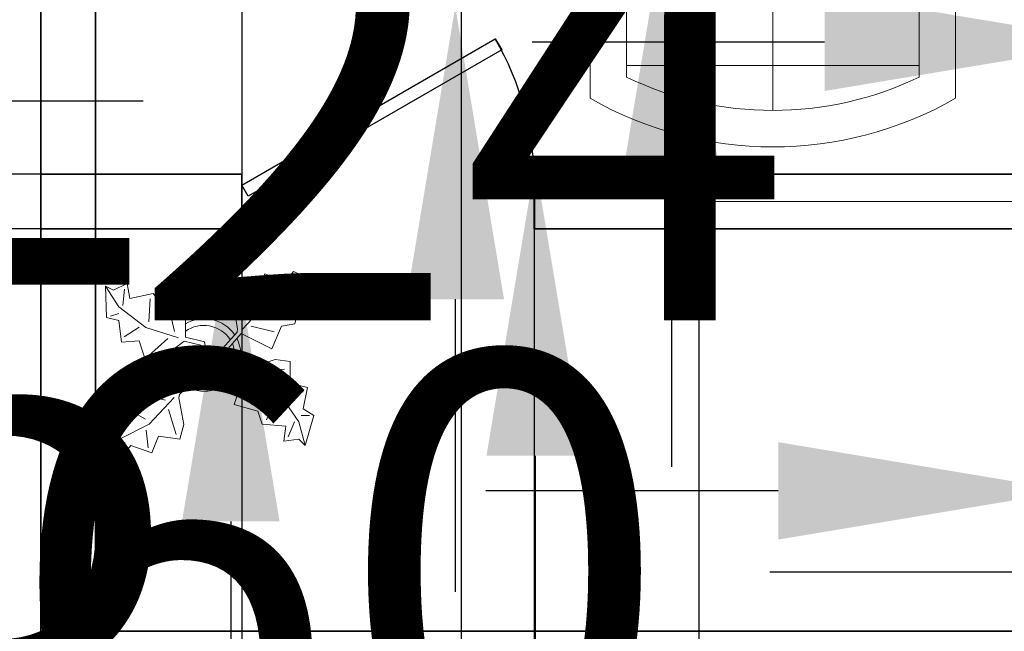
# Model space of a CAD drawing. Units: inches. Extents: x -307 to 2141, y -58 to 895.
# Tile 5 of 28: x 553 to 714, y 100 to 201. Entities that reach past the tile are written whole.
import ezdxf

# ---------------------------------------------------------------- set-up
doc = ezdxf.new("R2010")
doc.units = ezdxf.units.IN
doc.header["$MEASUREMENT"] = 0
for name, color, linetype, lineweight in [('A-ANNO-DIMS', 2, 'Continuous', 18), ('A-DOOR', 3, 'Continuous', 25), ('A-FURN', 8, 'Continuous', 18), ('A-GLAZ', 4, 'Continuous', 18), ('A-WALL', 7, 'Continuous', 35), ('L-PLNT', 94, 'Continuous', 13)]:
    doc.layers.add(name, color=color, linetype=linetype, lineweight=lineweight)
doc.styles.get("Standard").update_dxf_attribs({"font": 'arial.ttf'})
doc.dimstyles.get("Standard").update_dxf_attribs({"dimtxt": 72, "dimasz": 48, "dimexe": 0.18, "dimexo": 0.0625, "dimgap": 0.09, "dimtad": 0, "dimtih": 1, "dimtoh": 1, "dimdec": 0, "dimrnd": 48, "dimzin": 0, "dimdsep": 46, "dimlunit": 3, "dimtxsty": 'Standard', "dimcen": 0.09, "dimadec": 0, "dimazin": 0, "dimtfac": 1, "dimtdec": 0, "dimtofl": 0, "dimtmove": 0, "dimatfit": 3, "dimfxl": 1, "dimtolj": 1, "dimtzin": 0, "dimarcsym": 0})

# ---------------------------------------------------------------- blocks, each defined once
blk = doc.blocks.new('*U7')
for p, q in [((-40, 0), (-40, 6)), ((0, 0), (0, 6))]:
    blk.add_line(p, q)
blk.add_lwpolyline([(0, 0), (-34.64, -20), (-35.52, -18.48), (-0.88, 1.52)], close=True)
blk.add_arc((0, 0), 40, 180, 210)
blk = doc.blocks.new('Sofa - Roundback Loveseat 5 ft.')
for p, q in [((0, -32.44198), (0, -5.99998)), ((-24, -33.99998), (-24, -11.46958)), ((24.00004, -33.99998), (24.00004, -11.46958)), ((-23.9998, -13.38178), (23.99986, -13.38178)), ((-24, -32.44198), (24.00004, -32.44198))]:
    blk.add_line(p, q)
for points in [[(-24, -33.99998), (-30, -33.99998), (-30, -7.99998)], [(30.00004, -7.99998), (30.00004, -33.99998), (24.00004, -33.99998)]]:
    blk.add_lwpolyline(points)
for centre, radius, start, end in [((0, -60.24998), 60.24998, 60.13715, 119.8628), ((0, -61.38438), 55.38444, 64.32083, 115.6792)]:
    blk.add_arc(centre, radius, start, end)
blk = doc.blocks.new('Plant - Rubber or Philodendron')
for p, q in [((8.8871, 10.7908), (9.9809, 13.4933)), ((9.9809, 13.4933), (13.3837, 12.301)), ((13.3837, 12.301), (14.68, 13.9039)), ((14.5816, 13.2037), (14.3848, 11.8033)), ((14.68, 13.9039), (19.3848, 11.8146)), ((-16.2005, 11.4774), (-13.9899, 8.1064)), ((-16.2005, 11.4774), (-14.8639, 10.7964)), ((-16.0159, 6.3329), (-16.2005, 11.4774)), ((-14.8639, 10.7964), (-12.6195, 11.8975)), ((-12.6195, 11.8975), (-12.1909, 9.4345)), ((10.5828, 12.6946), (10.8893, 9.7953)), ((19.3848, 11.8146), (15.3859, 11.3055)), ((19.3848, 11.8146), (18.1868, 10.9119)), ((-13.3174, 8.325), (-13.0735, 11.0065)), ((-12.1909, 9.4345), (-8.3829, 10.3)), ((-8.3829, 10.3), (-7.0549, 8.501)), ((4.6914, 8.8812), (5.3859, 11.2828)), ((5.3859, 11.2828), (8.8871, 10.7908)), ((5.9878, 10.4842), (7.1971, 6.3869)), ((15.3859, 11.3055), (10.3916, 8.7942)), ((15.2875, 10.6053), (17.5907, 9.2105)), ((18.1868, 10.9119), (18.1925, 8.4119)), ((-13.9899, 8.1064), (-9.5434, 4.7185)), ((-8.8369, 9.409), (-9.0894, 5.6095)), ((-7.0549, 8.501), (-3.0284, 8.6941)), ((-3.0284, 8.6941), (-3.0709, 3.1041)), ((4.6914, 8.8812), (5.5014, 4.4831)), ((10.3916, 8.7942), (6.2847, 4.4028)), ((15.7909, 9.1065), (14.8995, 5.3044)), ((18.1925, 8.4119), (15.7909, 9.1065)), ((-15.3434, 6.5514), (-13.9984, 6.9884)), ((-4.8529, 4.012), (-5.7184, 7.82)), ((14.2977, 6.1031), (10.9934, 7.9956)), ((-14.0069, 5.8704), (-16.0159, 6.3329)), ((-13.5868, 2.2894), (-14.0069, 5.8704)), ((7.7005, 4.8881), (11.5025, 3.9967)), ((12.7005, 4.8994), (11.1089, 1.1958)), ((14.8995, 5.3044), (12.7005, 4.8994)), ((-13.1329, 3.1804), (-10.6614, 4.727)), ((-9.5434, 4.7185), (-4.1917, 2.9888)), ((2.1141, 0.2298), (5.4346, 3.9146)), ((6.1032, 3.6844), (2.8262, -0.031)), ((5.4346, 3.9146), (5.5014, 4.4831)), ((11.1089, 1.1958), (6.1032, 3.6844)), ((-10.6784, 2.491), (-13.5868, 2.2894)), ((-9.5858, -0.8715), (-10.6784, 2.491)), ((-9.1318, 0.0195), (-5.9793, 2.9025)), ((-7.1228, -0.443), (-3.5248, 2.2131)), ((-3.5248, 2.2131), (-3.3011, 2.4355)), ((-3.3011, 2.4355), (-0.5306, 1.7947)), ((-3.0709, 3.1041), (0.0797, 2.3163)), ((-0.5306, 1.7947), (-0.2255, -0.5527)), ((-0.5306, 1.7947), (-0.5306, 1.7947)), ((0.0797, 2.3163), (0.4866, -0.031)), ((0.4866, -0.031), (2.1141, 0.2298)), ((-7.1228, -0.443), (-9.5858, -0.8715)), ((-2.019, -3.6148), (-0.2255, -0.5527)), ((-0.9375, -3.1608), (0.5883, -0.8135)), ((0.5883, -0.8135), (2.2447, -2.0916)), ((2.8262, -0.031), (1.3003, -0.5527)), ((1.3003, -0.5527), (2.4193, -1.4655)), ((2.4193, -1.4655), (6.895, -2.1175)), ((11.6605, -0.5413), (6.895, -2.1175)), ((11.6605, -0.5413), (14.1354, -0.8948)), ((14.1354, -0.8948), (14.1354, -4.4304)), ((-4.0579, -6.2781), (-0.9375, -3.1608)), ((2.2447, -2.0916), (6.7108, -2.6626)), ((4.943, -7.9659), (6.7108, -2.6626)), ((12.3677, -6.1981), (7.219, -2.6772)), ((8.3544, -2.7453), (13.1973, -2.1704)), ((-11.3237, -7.2629), (-9.7321, -3.5593)), ((-9.7321, -3.5593), (-4.7264, -6.0479)), ((-2.019, -3.6148), (-4.7264, -6.0479)), ((8.125, -4.0768), (7.7715, -7.9659)), ((14.1354, -4.4304), (16.9638, -5.1375)), ((-6.3237, -7.2516), (-10.1257, -6.3602)), ((-4.1246, -6.8466), (-4.0579, -6.2781)), ((15.5496, -10.7943), (12.3677, -6.1981)), ((16.2567, -5.8446), (13.4283, -6.5517)), ((16.9638, -5.1375), (16.2567, -8.673)), ((-14.4141, -11.4699), (-13.5228, -7.6679)), ((-13.5228, -7.6679), (-11.3237, -7.2629)), ((-9.0148, -11.1577), (-4.9047, -6.8122)), ((-3.3146, -11.2447), (-4.1246, -6.8466)), ((8.8321, -9.0266), (4.943, -7.9659)), ((10.2463, -10.4408), (11.6605, -6.9053)), ((-12.921, -8.4665), (-9.6166, -10.359)), ((-4.611, -12.8477), (-5.8203, -8.7504)), ((9.5392, -11.1479), (8.8321, -9.0266)), ((16.2567, -8.673), (18.0245, -9.7337)), ((-16.8157, -10.7754), (-14.4141, -11.4699)), ((-16.8101, -13.2754), (-16.8157, -10.7754)), ((-14.0091, -13.669), (-9.0148, -11.1577)), ((-3.3146, -11.2447), (-4.0092, -13.6463)), ((13.4283, -11.5015), (9.5392, -11.1479)), ((14.8425, -10.7943), (13.7819, -13.2692)), ((16.6103, -14.6834), (15.5496, -10.7943)), ((17.3174, -9.7337), (15.9032, -9.7337)), ((18.0245, -9.7337), (16.6103, -14.6834)), ((-13.9107, -12.9688), (-16.2139, -11.574)), ((-9.206, -15.0581), (-9.5126, -12.1588)), ((13.0748, -13.9763), (13.4283, -11.5015)), ((-18.008, -14.1781), (-16.8101, -13.2754)), ((-18.008, -14.1781), (-14.0091, -13.669)), ((-13.3032, -16.2674), (-18.008, -14.1781)), ((-13.2048, -15.5672), (-13.008, -14.1668)), ((-7.5103, -13.1543), (-8.6042, -15.8568)), ((-4.0092, -13.6463), (-7.5103, -13.1543)), ((15.5496, -13.6228), (13.0748, -13.9763)), ((16.6103, -14.6834), (15.5496, -13.6228)), ((-12.0069, -14.6645), (-13.3032, -16.2674)), ((-8.6042, -15.8568), (-12.0069, -14.6645))]:
    blk.add_line(p, q)
for centre, radius, start, end in [((0, 0), 6.1275, 34.37569, 120.1028), ((-0.0601, -0.2075), 5.2461, 33.82192, 124.9414), ((-0.2664, 0.1682), 5.2775, 338.4094, 20.03007), ((-0.098, 0.1364), 6.1288, 341.2017, 26.09184), ((0.0308, 0.1664), 6, 178.6147, 235.1169), ((0.0308, 0.1664), 5, 168.1647, 238.6725), ((-0.0234, 0.3825), 6.1492, 242.5812, 331.2714), ((-0.1102, 0.4886), 5.2883, 247.3711, 327.472)]:
    blk.add_arc(centre, radius, start, end)
blk = doc.blocks.new('WIN-36IN-PAIR')
for p, q in [((72.02, 9), (72.02, 0)), ((0, 4.5), (36, 4.5)), ((36.02, 4.5), (72.02, 4.5))]:
    blk.add_line(p, q)
for points in [[(36, 0), (0, 0), (0, 9), (36, 9)], [(36.02, 9), (72.02, 9)], [(72.02, 0), (36.02, 0)]]:
    blk.add_lwpolyline(points)
blk = doc.blocks.new('*D28')
at = {"layer": 'A-ANNO-DIMS', "color": 0, "lineweight": -2, "transparency": 16777216}
for p, q in [((795.36, 433.55), (777.92, 433.55)), ((778.1, 385.55), (778.1, 366.07)), ((795.36, 318.07), (777.92, 318.07)), ((778.1, 318.07), (778.1, 270.07)), ((778.1, 270.07), (730.1, 270.07))]:
    blk.add_line(p, q, dxfattribs=at)
at = {"layer": 'A-ANNO-DIMS', "color": 0, "transparency": 16777216}
for points in [[(770.1, 385.55), (786.1, 385.55), (778.1, 433.55)], [(770.1, 366.07), (786.1, 366.07), (778.1, 318.07)]]:
    blk.add_solid(points, dxfattribs=at)
at = {"layer": 'Defpoints', "color": 0, "transparency": 16777216}
for p in [(795.42, 433.55), (778.1, 318.07), (795.42, 318.07)]:
    blk.add_point(p, dxfattribs=at)
at = {"layer": 'A-ANNO-DIMS', "color": 0, "transparency": 16777216, "insert": (534.42, 270.07), "char_height": 72, "attachment_point": 5}
blk.add_mtext('\\A1;BED 115', dxfattribs=at)
blk = doc.blocks.new('*D38')
at = {"layer": 'A-ANNO-DIMS', "color": 0, "lineweight": -2, "transparency": 16777216}
for p, q in [((598.5, 222.79), (550.5, 222.79)), ((646.5, 213.85), (646.5, 222.97)), ((706.5, 213.85), (706.5, 222.97)), ((754.5, 222.79), (802.5, 222.79))]:
    blk.add_line(p, q, dxfattribs=at)
at = {"layer": 'A-ANNO-DIMS', "color": 0, "transparency": 16777216}
for points in [[(598.5, 230.79), (598.5, 214.79), (646.5, 222.79)], [(754.5, 230.79), (754.5, 214.79), (706.5, 222.79)]]:
    blk.add_solid(points, dxfattribs=at)
at = {"layer": 'Defpoints', "color": 0, "transparency": 16777216}
for p in [(646.5, 222.79), (646.5, 213.79), (706.5, 213.79)]:
    blk.add_point(p, dxfattribs=at)
at = {"layer": 'A-ANNO-DIMS', "color": 0, "transparency": 16777216, "insert": (97.26, 222.79), "char_height": 72, "attachment_point": 5}
blk.add_mtext('\\A1;LOVESEAT 60 TYP.', dxfattribs=at)
blk = doc.blocks.new('*D39')
at = {"layer": 'A-ANNO-DIMS', "color": 0, "lineweight": -2, "transparency": 16777216}
for p, q in [((637.5, 261.79), (637.5, 309.79)), ((646.43, 213.79), (637.32, 213.79)), ((646.43, 177.12), (637.32, 177.12)), ((637.5, 129.12), (637.5, 81.12)), ((637.5, 81.12), (589.5, 81.12))]:
    blk.add_line(p, q, dxfattribs=at)
at = {"layer": 'A-ANNO-DIMS', "color": 0, "transparency": 16777216}
for points in [[(629.5, 261.79), (645.5, 261.79), (637.5, 213.79)], [(629.5, 129.12), (645.5, 129.12), (637.5, 177.12)]]:
    blk.add_solid(points, dxfattribs=at)
at = {"layer": 'Defpoints', "color": 0, "transparency": 16777216}
for p in [(646.5, 213.79), (637.5, 177.12), (646.5, 177.12)]:
    blk.add_point(p, dxfattribs=at)
at = {"layer": 'A-ANNO-DIMS', "color": 0, "transparency": 16777216, "insert": (414.2, 81.12), "char_height": 72, "attachment_point": 5}
blk.add_mtext('\\A1;37 TYP.', dxfattribs=at)
blk = doc.blocks.new('*D40')
at = {"layer": 'A-ANNO-DIMS', "color": 0, "lineweight": -2, "transparency": 16777216}
for p, q in [((725.38, 128.89), (725.38, 123.17)), ((762.77, 128.89), (762.77, 123.17)), ((677.38, 123.35), (629.38, 123.35)), ((810.77, 123.35), (858.77, 123.35))]:
    blk.add_line(p, q, dxfattribs=at)
at = {"layer": 'A-ANNO-DIMS', "color": 0, "transparency": 16777216}
for points in [[(677.38, 131.35), (677.38, 115.35), (725.38, 123.35)], [(810.77, 131.35), (810.77, 115.35), (762.77, 123.35)]]:
    blk.add_solid(points, dxfattribs=at)
at = {"layer": 'Defpoints', "color": 0, "transparency": 16777216}
for p in [(725.38, 128.96), (762.77, 128.96), (762.77, 123.35)]:
    blk.add_point(p, dxfattribs=at)
at = {"layer": 'A-ANNO-DIMS', "color": 0, "transparency": 16777216, "insert": (1208.37, 123.35), "char_height": 72, "attachment_point": 5}
blk.add_mtext('\\A1;PLANT 37 TYP.', dxfattribs=at)
blk = doc.blocks.new('*D48')
at = {"layer": 'A-ANNO-DIMS', "color": 0, "lineweight": -2, "transparency": 16777216}
for p, q in [((724, 313.98), (724, 361.98)), ((732.94, 265.98), (723.82, 265.98)), ((732.94, 205.98), (723.82, 205.98)), ((724, 157.98), (724, 109.98)), ((724, 109.98), (676, 109.98))]:
    blk.add_line(p, q, dxfattribs=at)
at = {"layer": 'A-ANNO-DIMS', "color": 0, "transparency": 16777216}
for points in [[(716, 313.98), (732, 313.98), (724, 265.98)], [(716, 157.98), (732, 157.98), (724, 205.98)]]:
    blk.add_solid(points, dxfattribs=at)
at = {"layer": 'Defpoints', "color": 0, "transparency": 16777216}
for p in [(733, 265.98), (724, 205.98), (733, 205.98)]:
    blk.add_point(p, dxfattribs=at)
at = {"layer": 'A-ANNO-DIMS', "color": 0, "transparency": 16777216, "insert": (321.56, 109.98), "char_height": 72, "attachment_point": 5}
blk.add_mtext('\\A1;MEDIA UNIT 60', dxfattribs=at)
blk = doc.blocks.new('*D49')
at = {"layer": 'A-ANNO-DIMS', "color": 0, "lineweight": -2, "transparency": 16777216}
for p, q in [((733, 205.92), (733, 196.8)), ((754.34, 205.92), (754.34, 196.8)), ((685, 196.98), (637, 196.98)), ((802.34, 196.98), (850.34, 196.98))]:
    blk.add_line(p, q, dxfattribs=at)
at = {"layer": 'A-ANNO-DIMS', "color": 0, "transparency": 16777216}
for points in [[(685, 204.98), (685, 188.98), (733, 196.98)], [(802.34, 204.98), (802.34, 188.98), (754.34, 196.98)]]:
    blk.add_solid(points, dxfattribs=at)
at = {"layer": 'Defpoints', "color": 0, "transparency": 16777216}
for p in [(733, 205.98), (754.34, 205.98), (754.34, 196.98)]:
    blk.add_point(p, dxfattribs=at)
at = {"layer": 'A-ANNO-DIMS', "color": 0, "transparency": 16777216, "insert": (895.66, 196.98), "char_height": 72, "attachment_point": 5}
blk.add_mtext('\\A1;21', dxfattribs=at)
blk = doc.blocks.new('*D58')
at = {"layer": 'A-ANNO-DIMS', "color": 0, "lineweight": -2, "transparency": 16777216}
for p, q in [((624.38, 334.8), (624.38, 382.8)), ((611.84, 286.8), (624.56, 286.8)), ((611.84, 202.8), (624.56, 202.8)), ((624.38, 154.8), (624.38, 106.8))]:
    blk.add_line(p, q, dxfattribs=at)
at = {"layer": 'A-ANNO-DIMS', "color": 0, "transparency": 16777216}
for points in [[(616.38, 334.8), (632.38, 334.8), (624.38, 286.8)], [(616.38, 154.8), (632.38, 154.8), (624.38, 202.8)]]:
    blk.add_solid(points, dxfattribs=at)
at = {"layer": 'Defpoints', "color": 0, "transparency": 16777216}
for p in [(611.78, 286.8), (624.38, 286.8), (611.78, 202.8)]:
    blk.add_point(p, dxfattribs=at)
at = {"layer": 'A-ANNO-DIMS', "color": 0, "transparency": 16777216, "insert": (624.38, 244.8), "char_height": 72, "attachment_point": 5}
blk.add_mtext('\\A1;SOFA 84', dxfattribs=at)
blk = doc.blocks.new('*D60')
at = {"layer": 'A-ANNO-DIMS', "color": 0, "lineweight": -2, "transparency": 16777216}
for p, q in [((659.86, 294.95), (659.86, 342.95)), ((659.86, 342.95), (707.86, 342.95)), ((663.34, 246.95), (659.68, 246.95)), ((663.34, 223.32), (659.68, 223.32)), ((659.86, 175.32), (659.86, 127.32))]:
    blk.add_line(p, q, dxfattribs=at)
at = {"layer": 'A-ANNO-DIMS', "color": 0, "transparency": 16777216}
for points in [[(651.86, 294.95), (667.86, 294.95), (659.86, 246.95)], [(651.86, 175.32), (667.86, 175.32), (659.86, 223.32)]]:
    blk.add_solid(points, dxfattribs=at)
at = {"layer": 'Defpoints', "color": 0, "transparency": 16777216}
for p in [(659.86, 246.95), (663.4, 246.95), (663.4, 223.32)]:
    blk.add_point(p, dxfattribs=at)
at = {"layer": 'A-ANNO-DIMS', "color": 0, "transparency": 16777216, "insert": (933.57, 342.95), "char_height": 72, "attachment_point": 5}
blk.add_mtext('\\A1;TABLE 24', dxfattribs=at)
blk = doc.blocks.new('*D63')
at = {"layer": 'A-ANNO-DIMS', "color": 0, "lineweight": -2, "transparency": 16777216}
for p, q in [((916.4, 691.34), (947.72, 691.34)), ((947.54, 643.34), (947.54, 416.19)), ((947.54, 115.34), (947.54, 342.49)), ((704.68, 67.34), (947.72, 67.34))]:
    blk.add_line(p, q, dxfattribs=at)
at = {"layer": 'A-ANNO-DIMS', "color": 0, "transparency": 16777216}
for points in [[(939.54, 643.34), (955.54, 643.34), (947.54, 691.34)], [(939.54, 115.34), (955.54, 115.34), (947.54, 67.34)]]:
    blk.add_solid(points, dxfattribs=at)
at = {"layer": 'Defpoints', "color": 0, "transparency": 16777216}
for p in [(916.34, 691.34), (704.62, 67.34), (947.54, 67.34)]:
    blk.add_point(p, dxfattribs=at)
at = {"layer": 'A-ANNO-DIMS', "color": 0, "transparency": 16777216, "insert": (947.54, 379.34), "char_height": 72, "attachment_point": 5}
blk.add_mtext('\\A1;624', dxfattribs=at)
blk = doc.blocks.new('*D64')
at = {"layer": 'A-ANNO-DIMS', "color": 0, "lineweight": -2, "transparency": 16777216}
for p, q in [((556.27, 691.34), (524.95, 691.34)), ((525.13, 643.34), (525.13, 465.69)), ((525.13, 214.34), (525.13, 391.99)), ((556.27, 166.34), (524.95, 166.34))]:
    blk.add_line(p, q, dxfattribs=at)
at = {"layer": 'A-ANNO-DIMS', "color": 0, "transparency": 16777216}
for points in [[(517.13, 643.34), (533.13, 643.34), (525.13, 691.34)], [(517.13, 214.34), (533.13, 214.34), (525.13, 166.34)]]:
    blk.add_solid(points, dxfattribs=at)
at = {"layer": 'Defpoints', "color": 0, "transparency": 16777216}
for p in [(525.13, 691.34), (556.34, 691.34), (556.34, 166.34)]:
    blk.add_point(p, dxfattribs=at)
at = {"layer": 'A-ANNO-DIMS', "color": 0, "transparency": 16777216, "insert": (525.13, 428.84), "char_height": 72, "attachment_point": 5}
blk.add_mtext('\\A1;525', dxfattribs=at)
blk = doc.blocks.new('*D65')
at = {"layer": 'A-ANNO-DIMS', "color": 0, "lineweight": -2, "transparency": 16777216}
for p, q in [((587.54, 252.57), (587.54, 300.57)), ((556.4, 204.57), (587.72, 204.57)), ((556.4, 166.34), (587.72, 166.34)), ((587.54, 118.34), (587.54, 70.34)), ((587.54, 70.34), (539.54, 70.34))]:
    blk.add_line(p, q, dxfattribs=at)
at = {"layer": 'A-ANNO-DIMS', "color": 0, "transparency": 16777216}
for points in [[(579.54, 252.57), (595.54, 252.57), (587.54, 204.57)], [(579.54, 118.34), (595.54, 118.34), (587.54, 166.34)]]:
    blk.add_solid(points, dxfattribs=at)
at = {"layer": 'Defpoints', "color": 0, "transparency": 16777216}
for p in [(556.34, 204.57), (556.34, 166.34), (587.54, 166.34)]:
    blk.add_point(p, dxfattribs=at)
at = {"layer": 'A-ANNO-DIMS', "color": 0, "transparency": 16777216, "insert": (417.99, 70.34), "char_height": 72, "attachment_point": 5}
blk.add_mtext('\\A1;38.23', dxfattribs=at)
blk = doc.blocks.new('*D66')
at = {"layer": 'A-ANNO-DIMS', "color": 0, "lineweight": -2, "transparency": 16777216}
for p, q in [((525.13, 382.34), (525.13, 430.34)), ((556.27, 334.34), (524.95, 334.34)), ((565.27, 304.34), (524.95, 304.34)), ((525.13, 256.34), (525.13, 208.34)), ((525.13, 208.34), (477.13, 208.34))]:
    blk.add_line(p, q, dxfattribs=at)
at = {"layer": 'A-ANNO-DIMS', "color": 0, "transparency": 16777216}
for points in [[(517.13, 382.34), (533.13, 382.34), (525.13, 334.34)], [(517.13, 256.34), (533.13, 256.34), (525.13, 304.34)]]:
    blk.add_solid(points, dxfattribs=at)
at = {"layer": 'Defpoints', "color": 0, "transparency": 16777216}
for p in [(556.34, 334.34), (525.13, 304.34), (565.34, 304.34)]:
    blk.add_point(p, dxfattribs=at)
at = {"layer": 'A-ANNO-DIMS', "color": 0, "transparency": 16777216, "insert": (425.62, 208.34), "char_height": 72, "attachment_point": 5}
blk.add_mtext('\\A1;30', dxfattribs=at)
blk = doc.blocks.new('*D70')
at = {"layer": 'A-ANNO-DIMS', "color": 0, "lineweight": -2, "transparency": 16777216}
for p, q in [((525.13184, 214.340828), (525.13184, 262.340828)), ((556.27334, 166.340828), (524.95184, 166.340828)), ((556.27334, 91.340828), (524.95184, 91.340828)), ((525.13184, 43.340828), (525.13184, -4.659172))]:
    blk.add_line(p, q, dxfattribs=at)
at = {"layer": 'A-ANNO-DIMS', "color": 0, "transparency": 16777216}
for points in [[(517.13184, 214.340828), (533.13184, 214.340828), (525.13184, 166.340828)], [(517.13184, 43.340828), (533.13184, 43.340828), (525.13184, 91.340828)]]:
    blk.add_solid(points, dxfattribs=at)
at = {"layer": 'Defpoints', "color": 0, "transparency": 16777216}
for p in [(525.13184, 166.340828), (556.33584, 166.340828), (556.33584, 91.340828)]:
    blk.add_point(p, dxfattribs=at)
at = {"layer": 'A-ANNO-DIMS', "color": 0, "transparency": 16777216, "insert": (525.13184, 128.840828), "char_height": 72, "attachment_point": 5}
blk.add_mtext('\\A1;75', dxfattribs=at)
blk = doc.blocks.new('*D71')
at = {"layer": 'A-ANNO-DIMS', "color": 0, "lineweight": -2, "transparency": 16777216}
for p, q in [((525.13, 139.34), (525.13, 187.34)), ((525.13, 187.34), (573.13, 187.34)), ((632.56, 91.34), (524.95, 91.34)), ((632.56, 67.34), (524.95, 67.34)), ((525.13, 19.34), (525.13, -28.66))]:
    blk.add_line(p, q, dxfattribs=at)
at = {"layer": 'A-ANNO-DIMS', "color": 0, "transparency": 16777216}
for points in [[(517.13, 139.34), (533.13, 139.34), (525.13, 91.34)], [(517.13, 19.34), (533.13, 19.34), (525.13, 67.34)]]:
    blk.add_solid(points, dxfattribs=at)
at = {"layer": 'Defpoints', "color": 0, "transparency": 16777216}
for p in [(525.13, 91.34), (632.62, 91.34), (632.62, 67.34)]:
    blk.add_point(p, dxfattribs=at)
at = {"layer": 'A-ANNO-DIMS', "color": 0, "transparency": 16777216, "insert": (625.26, 187.34), "char_height": 72, "attachment_point": 5}
blk.add_mtext('\\A1;24', dxfattribs=at)
blk = doc.blocks.new('*D86')
at = {"layer": 'A-ANNO-DIMS', "color": 0, "lineweight": -2, "transparency": 16777216}
for p, q in [((565.34, 304.28), (565.34, 35.96)), ((625.34, 304.28), (625.34, 35.96)), ((517.34, 36.14), (469.34, 36.14)), ((673.34, 36.14), (721.34, 36.14))]:
    blk.add_line(p, q, dxfattribs=at)
at = {"layer": 'A-ANNO-DIMS', "color": 0, "transparency": 16777216}
for points in [[(517.34, 44.14), (517.34, 28.14), (565.34, 36.14)], [(673.34, 44.14), (673.34, 28.14), (625.34, 36.14)]]:
    blk.add_solid(points, dxfattribs=at)
at = {"layer": 'Defpoints', "color": 0, "transparency": 16777216}
for p in [(565.34, 304.34), (625.34, 304.34), (625.34, 36.14)]:
    blk.add_point(p, dxfattribs=at)
at = {"layer": 'A-ANNO-DIMS', "color": 0, "transparency": 16777216, "insert": (773.07, 36.14), "char_height": 72, "attachment_point": 5}
blk.add_mtext('\\A1;60', dxfattribs=at)
blk = doc.blocks.new('*D89')
at = {"layer": 'A-ANNO-DIMS', "color": 0, "lineweight": -2, "transparency": 16777216}
for p, q in [((525.13, 295.34), (525.13, 343.34)), ((525.13, 343.34), (573.13, 343.34)), ((565.27, 295.34), (524.95, 295.34)), ((525.13, 223.34), (525.13, 247.34)), ((556.27, 175.34), (524.95, 175.34))]:
    blk.add_line(p, q, dxfattribs=at)
at = {"layer": 'A-ANNO-DIMS', "color": 0, "transparency": 16777216}
for points in [[(517.13, 247.34), (533.13, 247.34), (525.13, 295.34)], [(517.13, 223.34), (533.13, 223.34), (525.13, 175.34)]]:
    blk.add_solid(points, dxfattribs=at)
at = {"layer": 'Defpoints', "color": 0, "transparency": 16777216}
for p in [(525.13, 295.34), (565.34, 295.34), (556.34, 175.34)]:
    blk.add_point(p, dxfattribs=at)
at = {"layer": 'A-ANNO-DIMS', "color": 0, "transparency": 16777216, "insert": (649.25, 343.34), "char_height": 72, "attachment_point": 5}
blk.add_mtext('\\A1;120', dxfattribs=at)
blk = doc.blocks.new('*D90')
at = {"layer": 'A-ANNO-DIMS', "color": 0, "lineweight": -2, "transparency": 16777216}
for p, q in [((556.34, 166.28), (556.34, 35.96)), ((589.34, 166.28), (589.34, 35.96)), ((508.34, 36.14), (460.34, 36.14)), ((637.34, 36.14), (685.34, 36.14))]:
    blk.add_line(p, q, dxfattribs=at)
at = {"layer": 'A-ANNO-DIMS', "color": 0, "transparency": 16777216}
for points in [[(508.34, 44.14), (508.34, 28.14), (556.34, 36.14)], [(637.34, 44.14), (637.34, 28.14), (589.34, 36.14)]]:
    blk.add_solid(points, dxfattribs=at)
at = {"layer": 'Defpoints', "color": 0, "transparency": 16777216}
for p in [(556.34, 166.34), (589.34, 166.34), (589.34, 36.14)]:
    blk.add_point(p, dxfattribs=at)
at = {"layer": 'A-ANNO-DIMS', "color": 0, "transparency": 16777216, "insert": (736.97, 36.14), "char_height": 72, "attachment_point": 5}
blk.add_mtext('\\A1;33', dxfattribs=at)
blk = doc.blocks.new('*D91')
at = {"layer": 'A-ANNO-DIMS', "color": 0, "lineweight": -2, "transparency": 16777216}
for p, q in [((589.34, 166.28), (589.34, 35.96)), ((637.34, 166.28), (637.34, 35.96)), ((541.34, 36.14), (493.34, 36.14)), ((685.34, 36.14), (733.34, 36.14))]:
    blk.add_line(p, q, dxfattribs=at)
at = {"layer": 'A-ANNO-DIMS', "color": 0, "transparency": 16777216}
for points in [[(541.34, 44.14), (541.34, 28.14), (589.34, 36.14)], [(685.34, 44.14), (685.34, 28.14), (637.34, 36.14)]]:
    blk.add_solid(points, dxfattribs=at)
at = {"layer": 'Defpoints', "color": 0, "transparency": 16777216}
for p in [(589.34, 166.34), (637.34, 166.34), (637.34, 36.14)]:
    blk.add_point(p, dxfattribs=at)
at = {"layer": 'A-ANNO-DIMS', "color": 0, "transparency": 16777216, "insert": (786.52, 36.14), "char_height": 72, "attachment_point": 5}
blk.add_mtext('\\A1;48', dxfattribs=at)
blk = doc.blocks.new('*D92')
at = {"layer": 'A-ANNO-DIMS', "color": 0, "lineweight": -2, "transparency": 16777216}
for p, q in [((637.34, 166.28), (637.34, 35.96)), ((664.34, 166.28), (664.34, 35.96)), ((589.34, 36.14), (541.34, 36.14)), ((712.34, 36.14), (760.34, 36.14))]:
    blk.add_line(p, q, dxfattribs=at)
at = {"layer": 'A-ANNO-DIMS', "color": 0, "transparency": 16777216}
for points in [[(589.34, 44.14), (589.34, 28.14), (637.34, 36.14)], [(712.34, 44.14), (712.34, 28.14), (664.34, 36.14)]]:
    blk.add_solid(points, dxfattribs=at)
at = {"layer": 'Defpoints', "color": 0, "transparency": 16777216}
for p in [(637.34, 166.34), (664.34, 166.34), (664.34, 36.14)]:
    blk.add_point(p, dxfattribs=at)
at = {"layer": 'A-ANNO-DIMS', "color": 0, "transparency": 16777216, "insert": (812.61, 36.14), "char_height": 72, "attachment_point": 5}
blk.add_mtext('\\A1;27', dxfattribs=at)
blk = doc.blocks.new('*D99')
at = {"layer": 'A-ANNO-DIMS', "color": 0, "lineweight": -2, "transparency": 16777216}
for p, q in [((763.34, 481.28), (763.34, 35.96)), ((802.34, 481.28), (802.34, 35.96)), ((715.34, 36.14), (667.34, 36.14)), ((850.34, 36.14), (898.34, 36.14))]:
    blk.add_line(p, q, dxfattribs=at)
at = {"layer": 'A-ANNO-DIMS', "color": 0, "transparency": 16777216}
for points in [[(715.34, 44.14), (715.34, 28.14), (763.34, 36.14)], [(850.34, 44.14), (850.34, 28.14), (802.34, 36.14)]]:
    blk.add_solid(points, dxfattribs=at)
at = {"layer": 'Defpoints', "color": 0, "transparency": 16777216}
for p in [(763.34, 481.34), (802.34, 481.34), (802.34, 36.14)]:
    blk.add_point(p, dxfattribs=at)
at = {"layer": 'A-ANNO-DIMS', "color": 0, "transparency": 16777216, "insert": (950.04, 36.14), "char_height": 72, "attachment_point": 5}
blk.add_mtext('\\A1;39', dxfattribs=at)
blk = doc.blocks.new('*D100')
at = {"layer": 'A-ANNO-DIMS', "color": 0, "lineweight": -2, "transparency": 16777216}
for p, q in [((589.34, 409.28), (589.34, 35.96)), ((625.34, 409.28), (625.34, 35.96)), ((541.34, 36.14), (493.34, 36.14)), ((673.34, 36.14), (721.34, 36.14))]:
    blk.add_line(p, q, dxfattribs=at)
at = {"layer": 'A-ANNO-DIMS', "color": 0, "transparency": 16777216}
for points in [[(541.34, 44.14), (541.34, 28.14), (589.34, 36.14)], [(673.34, 44.14), (673.34, 28.14), (625.34, 36.14)]]:
    blk.add_solid(points, dxfattribs=at)
at = {"layer": 'Defpoints', "color": 0, "transparency": 16777216}
for p in [(589.34, 409.34), (625.34, 409.34), (625.34, 36.14)]:
    blk.add_point(p, dxfattribs=at)
at = {"layer": 'A-ANNO-DIMS', "color": 0, "transparency": 16777216, "insert": (772.95, 36.14), "char_height": 72, "attachment_point": 5}
blk.add_mtext('\\A1;36', dxfattribs=at)

msp = doc.modelspace()

# ---------------------------------------------------------------- linework, layer by layer
at = {"layer": 'A-WALL'}
for p, q in [((556.3358, 691.3408), (556.3358, 91.3408)), ((565.3358, 682.3408), (565.3358, 100.3408)), ((589.3358, 175.3408), (556.3358, 175.3408)), ((589.3358, 175.3408), (589.3358, 166.3408)), ((754.3358, 175.3408), (637.3358, 175.3408)), ((637.3358, 175.3408), (637.3358, 166.3408)), ((589.3358, 166.3408), (556.3358, 166.3408)), ((763.3358, 166.3408), (637.3358, 166.3408)), ((565.3358, 100.3408), (763.3358, 100.3408))]:
    msp.add_line(p, q, dxfattribs=at)

# ---------------------------------------------------------------- block references
at = {"layer": 'A-DOOR', "xscale": 1.201029199664418, "yscale": 1.201029199664418, "zscale": 1.201029199664418, "rotation": 179.9999999999999}
msp.add_blockref('*U7', (589.3358, 173.547), dxfattribs=at)
at = {"layer": 'A-FURN', "rotation": 180}
msp.add_blockref('Sofa - Roundback Loveseat 5 ft.', (676.4965, 179.7908), dxfattribs=at)
at = {"layer": 'A-GLAZ'}
msp.add_blockref('WIN-36IN-PAIR', (664.336, 166.341), dxfattribs=at)
at = {"layer": 'L-PLNT'}
msp.add_blockref('Plant - Rubber or Philodendron', (583.1583, 145.4681), dxfattribs=at)

# ---------------------------------------------------------------- dimensions: what is measured, and where the dimension line sits
at = {"layer": 'A-ANNO-DIMS'}
for base, p1, p2, angle, override, picture, middle in [((525.1318, 691.3408), (556.3358, 166.3408), (556.3358, 691.3408), 90, {"dimdec": 0, "dimlfac": 1, "dimrnd": 0, "dimzin": 0, "dimdsep": 46, "dimlunit": 2}, '*D64', (525.1318, 428.8408)), ((947.5398, 67.3408), (916.3358, 691.3408), (704.6211, 67.3408), 90, {"dimdec": 0, "dimlfac": 1, "dimrnd": 0, "dimzin": 0, "dimdsep": 46, "dimlunit": 2}, '*D63', (947.5398, 379.3408)), ((525.1318, 304.3408), (556.3358, 334.3416), (565.3358, 304.3408), 90, {"dimdec": 0, "dimlfac": 1, "dimrnd": 0, "dimzin": 0, "dimdsep": 46, "dimlunit": 2}, '*D66', (425.6203, 208.3408)), ((525.1318, 295.3408), (556.3358, 175.3408), (565.3358, 295.3408), 90, {"dimdec": 0, "dimlfac": 1, "dimrnd": 0, "dimzin": 0, "dimdsep": 46, "dimlunit": 2}, '*D89', (649.2491, 343.3408)), ((587.5398, 166.3408), (556.3358, 204.574), (556.3358, 166.3408), 270, {"dimdec": 2, "dimlfac": 1, "dimrnd": 0, "dimzin": 0, "dimdsep": 46, "dimlunit": 2}, '*D65', (417.9928, 70.3408)), ((525.1318, 166.3408), (556.3358, 91.3408), (556.3358, 166.3408), 90, {"dimdec": 0, "dimlfac": 1, "dimrnd": 0, "dimzin": 0, "dimdsep": 46, "dimlunit": 2}, '*D70', (525.1318, 128.8408)), ((525.1318, 91.3408), (632.6211, 67.3408), (632.6211, 91.3408), 90, {"dimdec": 0, "dimlfac": 1, "dimrnd": 0, "dimzin": 0, "dimdsep": 46, "dimlunit": 2}, '*D71', (625.2573, 187.3408))]:
    dim = msp.add_linear_dim(base=base, p1=p1, p2=p2, angle=angle, dimstyle='Standard', override=override, dxfattribs=at)
    dim.commit()
    dim.dimension.update_dxf_attribs({"geometry": picture, "text_midpoint": middle})
for base, p1, p2, picture, middle in [((802.3358, 36.1368), (763.3358, 481.3408), (802.3358, 481.3408), '*D99', (950.0438, 36.1368)), ((625.3358, 36.1368), (589.339, 409.3408), (625.3358, 409.3408), '*D100', (772.9456, 36.1368)), ((625.3358, 36.1368), (565.3358, 304.3408), (625.3358, 304.3408), '*D86', (773.0684, 36.1368)), ((754.3358, 196.9815), (733.0025, 205.9815), (754.3358, 205.9815), '*D49', (895.6591, 196.9815)), ((589.3358, 36.1368), (556.3358, 166.3408), (589.3358, 166.3408), '*D90', (736.9702, 36.1368)), ((637.3358, 36.1368), (589.3358, 166.3408), (637.3358, 166.3408), '*D91', (786.5172, 36.1368)), ((664.3358, 36.1368), (637.3358, 166.3408), (664.3358, 166.3408), '*D92', (812.6087, 36.1368))]:
    dim = msp.add_linear_dim(base=base, p1=p1, p2=p2, dimstyle='Standard', override={"dimdec": 0, "dimlfac": 1, "dimrnd": 0, "dimzin": 0, "dimdsep": 46, "dimlunit": 2}, dxfattribs=at)
    dim.commit()
    dim.dimension.update_dxf_attribs({"geometry": picture, "text_midpoint": middle})
for base, p1, p2, angle, text, picture, middle in [((659.8571, 246.9465), (663.4018, 223.3153), (663.4018, 246.9465), 90, 'TABLE <>', '*D60', (933.5733, 342.9465)), ((778.0993, 318.073), (795.4208, 433.5496), (795.4208, 318.073), 270, 'BED <>', '*D28', (534.4158, 270.073)), ((646.4965, 222.7908), (706.4965, 213.7908), (646.4965, 213.7908), 180, 'LOVESEAT <> TYP.', '*D38', (97.2632, 222.7908)), ((624.377, 286.7976), (611.777, 202.7976), (611.777, 286.7976), 90, 'SOFA <>', '*D58', (624.377, 244.7976)), ((724.0025, 205.9815), (733.0025, 265.9815), (733.0025, 205.9815), 270, 'MEDIA UNIT <>', '*D48', (321.5605, 109.9815)), ((637.4965, 177.1242), (646.4965, 213.7908), (646.4965, 177.1242), 270, '<> TYP.', '*D39', (414.195, 81.1242))]:
    dim = msp.add_linear_dim(base=base, p1=p1, p2=p2, angle=angle, text=text, dimstyle='Standard', override={"dimdec": 0, "dimlfac": 1, "dimrnd": 0, "dimzin": 0, "dimdsep": 46, "dimlunit": 2}, dxfattribs=at)
    dim.commit()
    dim.dimension.update_dxf_attribs({"geometry": picture, "text_midpoint": middle})
dim = msp.add_linear_dim(base=(762.7703, 123.348), p1=(725.3775, 128.9569), p2=(762.7703, 128.9569), text='PLANT <> TYP.', dimstyle='Standard', override={"dimdec": 0, "dimlfac": 1, "dimrnd": 0, "dimzin": 0, "dimdsep": 46, "dimlunit": 2}, dxfattribs=at)
dim.commit()
dim.dimension.update_dxf_attribs({"geometry": '*D40', "text_midpoint": (1208.3746, 123.348)})

doc.saveas('drawing.dxf')
